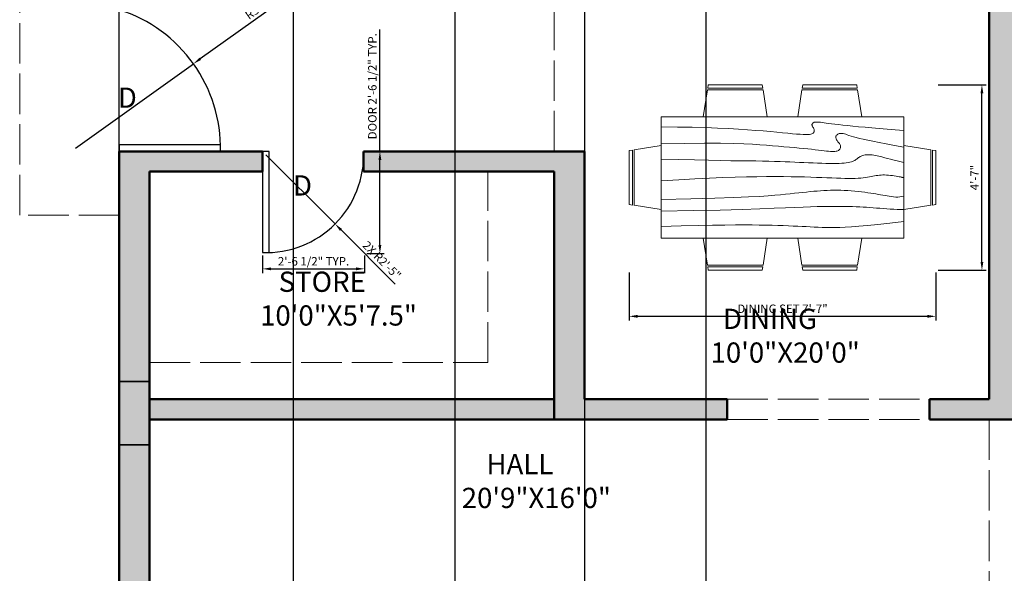
# Model space of a CAD drawing. Units: inches. Extents: x 5703 to 6226, y 10088 to 10813.
# Tile 3 of 5: x 5744 to 6036, y 10460 to 10624. Entities that reach past the tile are written whole.
import ezdxf

# ---------------------------------------------------------------- set-up
doc = ezdxf.new("R2010")
doc.units = ezdxf.units.IN
doc.linetypes.add('ACAD_ISO02W100', pattern=[15, 12, -3])
for name, color, linetype, lineweight in [('A-ANNO-DIMS', 2, 'Continuous', 18), ('A-ANNO-TEXT', 7, 'Continuous', 18), ('A-AREA-IDEN', 7, 'Continuous', 18), ('A-COLS', 7, 'Continuous', 35), ('A-COLS-PATT', 7, 'Continuous', 13), ('A-DOOR', 140, 'Continuous', 25), ('A-FURN', 8, 'Continuous', 18), ('A-WALL', 7, 'Continuous', 50), ('A-WALL-PATT', 9, 'Continuous', 13)]:
    doc.layers.add(name, color=color, linetype=linetype, lineweight=lineweight)
for name, color, linetype, lineweight, true_color in [('A-FLOR-CASE-OVHD', 30, 'ACAD_ISO02W100', 18, 0xf8991e), ('A-ROOF-OVHD', 30, 'ACAD_ISO02W100', 18, 0xf8991e), ('A-WALL-OVHD', 30, 'ACAD_ISO02W100', 18, 0xf8991e)]:
    doc.layers.add(name, color=color, linetype=linetype, lineweight=lineweight, true_color=true_color)
doc.styles.get("Standard").update_dxf_attribs({"font": 'arial.ttf'})
doc.dimstyles.new('ISO-25', dxfattribs={"dimtxt": 2.5, "dimasz": 2.5, "dimexe": 1.25, "dimexo": 0.625, "dimtad": 1, "dimlunit": 3, "dimtxsty": 'Standard', "dimcen": 2.5, "dimadec": 0, "dimazin": 0, "dimtfac": 1, "dimtmove": 0, "dimatfit": 3, "dimfxl": 1, "dimarcsym": 0})

# ---------------------------------------------------------------- blocks, each defined once
blk = doc.blocks.new('Dining Set - 36 x 72 in.')
for p, q in [((-22, 27.5), (-22.1562, 26.50042)), ((-5.8416, 26.5), (-22.1534, 26.5)), ((-22, 27.5), (-6, 27.5)), ((-5.8437, 26.49966), (-6, 27.5)), ((6, 27.5), (5.8438, 26.50042)), ((22.1584, 26.5), (5.8466, 26.5)), ((6, 27.5), (22, 27.5)), ((22.1563, 26.49966), (22, 27.5)), ((-22.2343, 26.00059), (-23.4847, 17.99762)), ((-22.2304, 26), (-5.7608, 26)), ((-4.5152, 17.99762), (-5.7655, 25.99926)), ((5.7657, 26.00059), (4.5153, 17.99762)), ((5.7696, 26), (22.2392, 26)), ((23.4848, 17.99762), (22.2345, 25.99926)), ((36, 18), (-36, 18)), ((-36, 18), (-36, -18)), ((36, -18), (36, 18)), ((-44.0006, 8.23428), (-35.9976, 9.48474)), ((44.0006, 8.23428), (35.9976, 9.48474)), ((-45.5, 8), (-44.5004, 8.15617)), ((-45.5, 8), (-45.5, -8)), ((-44.5, -8.15843), (-44.5, 8.15338)), ((-44, 8.23041), (-44, -8.23915)), ((44, 8.23041), (44, -8.23915)), ((44.5, -8.15843), (44.5, 8.15338)), ((45.5, 8), (44.5005, 8.15617)), ((45.5, 8), (45.5, -8)), ((-44.4997, -8.15631), (-45.5, -8)), ((-35.9976, -9.48476), (-43.9993, -8.2345)), ((35.9976, -9.48476), (43.9993, -8.2345)), ((44.4997, -8.15631), (45.5, -8)), ((-36, -18), (36, -18)), ((-22.2343, -26.0006), (-23.4847, -17.99762)), ((-4.5152, -17.99762), (-5.7655, -25.99928)), ((5.7657, -26.0006), (4.5153, -17.99762)), ((23.4848, -17.99762), (22.2345, -25.99928)), ((-22.2304, -26), (-5.7608, -26)), ((5.7696, -26), (22.2392, -26)), ((-22, -27.5), (-22.1562, -26.50044)), ((-5.8416, -26.5), (-22.1534, -26.5)), ((-22, -27.5), (-6, -27.5)), ((-5.8437, -26.49967), (-6, -27.5)), ((6, -27.5), (5.8438, -26.50044)), ((22.1584, -26.5), (5.8466, -26.5)), ((6, -27.5), (22, -27.5)), ((22.1563, -26.49967), (22, -27.5))]:
    blk.add_line(p, q)
for points in [[(-36, 15), (-31.1772, 14.97754), (-26.8079, 14.91406), (-22.8538, 14.81543), (-19.276, 14.6875), (-16.0362, 14.53613), (-13.0957, 14.36718), (-10.4159, 14.18652), (-7.9583, 14), (-5.6904, 13.81315), (-3.6035, 13.63021), (-1.6954, 13.45508), (0.0365, 13.29166), (1.5945, 13.14388), (2.9811, 13.01562), (4.1988, 12.9108), (5.25, 12.83333), (6.1393, 12.78613), (6.8802, 12.76823), (7.4883, 12.77767), (7.9792, 12.8125), (8.3685, 12.87077), (8.6719, 12.95052), (8.9049, 13.0498), (9.0833, 13.16666), (9.2205, 13.29899), (9.3216, 13.44401), (9.3895, 13.59879), (9.4271, 13.76041), (9.4373, 13.92594), (9.4232, 14.09245), (9.3875, 14.257), (9.3333, 14.41666), (9.2638, 14.56917), (9.1836, 14.71484), (9.0975, 14.85465), (9.0104, 14.98958), (8.9272, 15.1206), (8.8529, 15.2487), (8.7922, 15.37483), (8.75, 15.5), (8.7305, 15.62467), (8.7344, 15.74739), (8.7617, 15.86621), (8.8125, 15.97916), (8.8867, 16.08431), (8.9844, 16.17968), (9.1055, 16.26334), (9.25, 16.33333), (9.4189, 16.38802), (9.6172, 16.42708), (9.8506, 16.45052), (10.125, 16.45833), (10.4463, 16.45052), (10.8203, 16.42708), (11.2529, 16.38802), (11.75, 16.33333), (12.3184, 16.26318), (12.9694, 16.17838), (13.7151, 16.07991), (14.5677, 15.96875), (15.5395, 15.84586), (16.6426, 15.71224), (17.8893, 15.56884), (19.2917, 15.41666), (20.859, 15.25667), (22.5879, 15.08984), (24.4721, 14.91715), (26.5052, 14.73958), (28.6809, 14.5581), (30.9929, 14.3737), (33.4347, 14.18733), (36, 14)], [(-36, 10), (-28.9766, 10.14274), (-23.1725, 10.20442), (-18.4241, 10.19775), (-14.5677, 10.13541), (-11.4399, 10.03011), (-8.877, 9.89453), (-6.7154, 9.74137), (-4.7917, 9.58333), (-2.9698, 9.43082), (-1.2246, 9.28515), (0.4415, 9.14534), (2.026, 9.01041), (3.5266, 8.87939), (4.9408, 8.7513), (6.266, 8.62516), (7.5, 8.5), (8.6411, 8.37549), (9.6914, 8.2539), (10.6538, 8.13818), (11.5312, 8.03125), (12.3267, 7.93603), (13.043, 7.85547), (13.6831, 7.79248), (14.25, 7.75), (14.7471, 7.7303), (15.1797, 7.73307), (15.5537, 7.75732), (15.875, 7.80208), (16.1494, 7.86637), (16.3828, 7.94922), (16.5811, 8.04964), (16.75, 8.16666), (16.8944, 8.29915), (17.0143, 8.44531), (17.1089, 8.60319), (17.1771, 8.77083), (17.218, 8.94629), (17.2305, 9.1276), (17.2137, 9.31282), (17.1667, 9.5), (17.0895, 9.6875), (16.987, 9.875), (16.8649, 10.0625), (16.7292, 10.25), (16.5856, 10.4375), (16.4401, 10.625), (16.2985, 10.8125), (16.1667, 11), (16.05, 11.18733), (15.9518, 11.3737), (15.8752, 11.5581), (15.8229, 11.73958), (15.798, 11.91715), (15.8034, 12.08984), (15.842, 12.25667), (15.9167, 12.41666), (16.0295, 12.56836), (16.1784, 12.70833), (16.3605, 12.83268), (16.5729, 12.9375), (16.8127, 13.01888), (17.0768, 13.07291), (17.3625, 13.0957), (17.6667, 13.08333), (17.9894, 13.03312), (18.3418, 12.94726), (18.7382, 12.82918), (19.1927, 12.68229), (19.7195, 12.51001), (20.3327, 12.31575), (21.0465, 12.10294), (21.875, 11.875), (22.8357, 11.63354), (23.959, 11.37304), (25.2786, 11.08618), (26.8282, 10.76562), (28.6414, 10.40405), (30.752, 9.99414), (33.1936, 9.52856), (36, 9)], [(-36, 5.5), (-30.7157, 5.3348), (-26.069, 5.20963), (-21.9946, 5.11767), (-18.4271, 5.05208), (-15.3009, 5.00602), (-12.5508, 4.97265), (-10.1112, 4.94515), (-7.9167, 4.91666), (-5.909, 4.88167), (-4.0586, 4.83984), (-2.3429, 4.79215), (-0.7396, 4.73958), (0.7739, 4.6831), (2.22, 4.6237), (3.6213, 4.56233), (5, 4.5), (6.373, 4.43782), (7.7344, 4.3776), (9.0723, 4.32129), (10.375, 4.27083), (11.6309, 4.22819), (12.8281, 4.19531), (13.9551, 4.17415), (15, 4.16666), (15.954, 4.17448), (16.819, 4.19791), (17.6001, 4.23698), (18.3021, 4.29166), (18.9299, 4.36198), (19.4883, 4.44791), (19.9823, 4.54948), (20.4167, 4.66666), (20.7969, 4.79899), (21.1302, 4.94401), (21.4245, 5.09879), (21.6875, 5.26041), (21.9271, 5.42594), (22.1511, 5.59245), (22.3672, 5.757), (22.5834, 5.91666), (22.8065, 6.06868), (23.0404, 6.21093), (23.2879, 6.34147), (23.5521, 6.45833), (23.8358, 6.55957), (24.142, 6.64323), (24.4735, 6.70735), (24.8334, 6.75), (25.2235, 6.76969), (25.642, 6.76692), (26.0858, 6.74267), (26.5521, 6.69791), (27.0379, 6.63362), (27.5404, 6.55078), (28.0565, 6.45036), (28.5834, 6.33333), (29.1242, 6.19987), (29.7071, 6.04687), (30.3661, 5.87044), (31.1354, 5.66666), (32.0493, 5.43164), (33.142, 5.16146), (34.4475, 4.85221), (36, 4.5)], [(-36, -1), (-30.7915, -0.6591), (-26.0195, -0.38216), (-21.6519, -0.16284), (-17.6563, 0.00521), (-14.0005, 0.12833), (-10.6523, 0.21289), (-7.5796, 0.26522), (-4.75, 0.29166), (-2.134, 0.29793), (0.2878, 0.28711), (2.5317, 0.26163), (4.6146, 0.22396), (6.5529, 0.17651), (8.3633, 0.12174), (10.0623, 0.06209), (11.6667, 0), (13.1899, -0.06201), (14.6341, -0.1211), (15.9982, -0.17432), (17.2813, -0.21875), (18.4823, -0.25147), (19.6003, -0.26953), (20.6343, -0.27002), (21.5834, -0.25), (22.4481, -0.20768), (23.2357, -0.14584), (23.9549, -0.06836), (24.6146, 0.02083), (25.2235, 0.11784), (25.7904, 0.21875), (26.3241, 0.31966), (26.8334, 0.41666), (27.3265, 0.50618), (27.8099, 0.58593), (28.2894, 0.65397), (28.7709, 0.70833), (29.2601, 0.74707), (29.763, 0.76823), (30.2855, 0.76985), (30.8334, 0.75), (31.4088, 0.70784), (31.9994, 0.64713), (32.589, 0.57275), (33.1615, 0.48958), (33.7008, 0.4025), (34.1908, 0.3164), (34.6153, 0.23616), (34.9584, 0.16666), (35.2099, 0.11165), (35.3848, 0.07031), (35.504, 0.04069), (35.5886, 0.02083), (35.6594, 0.00879), (35.7377, 0.0026), (35.8442, 0.00032), (36, 0)], [(-36, -6.5), (-27.1843, -6.31267), (-20.084, -6.1263), (-14.469, -5.9419), (-10.1094, -5.76042), (-6.7752, -5.58285), (-4.2363, -5.41016), (-2.2629, -5.24333), (-0.625, -5.08334), (0.8708, -4.93099), (2.2715, -4.78646), (3.5872, -4.64974), (4.8281, -4.52084), (6.0046, -4.39974), (7.127, -4.28646), (8.2053, -4.18099), (9.25, -4.08334), (10.2705, -3.99382), (11.2734, -3.91407), (12.2647, -3.84603), (13.25, -3.79167), (14.2354, -3.75293), (15.2266, -3.73177), (16.2295, -3.73015), (17.25, -3.75), (18.2912, -3.79248), (19.3451, -3.85547), (20.4009, -3.93604), (21.4479, -4.03125), (22.4754, -4.13819), (23.4727, -4.25391), (24.4289, -4.37549), (25.3334, -4.5), (26.1785, -4.62492), (26.9694, -4.74935), (27.7145, -4.87281), (28.4219, -4.99479), (29.1, -5.11483), (29.7572, -5.23242), (30.4016, -5.34709), (31.0417, -5.45834), (31.6837, -5.56437), (32.3262, -5.65821), (32.9658, -5.73153), (33.599, -5.77604), (34.2224, -5.78345), (34.8327, -5.74545), (35.4264, -5.65373), (36, -5.5)], [(-36, -10), (-26.4022, -9.81299), (-18.4675, -9.62891), (-11.9839, -9.45069), (-6.7396, -9.28125), (-2.5226, -9.12354), (0.8789, -8.98047), (3.6769, -8.85498), (6.0833, -8.75), (8.2767, -8.66765), (10.3021, -8.60677), (12.1712, -8.56543), (13.8958, -8.54167), (15.4876, -8.53353), (16.9583, -8.53907), (18.3197, -8.55632), (19.5834, -8.58334), (20.7616, -8.61841), (21.8685, -8.66081), (22.9188, -8.71004), (23.9271, -8.76563), (24.9081, -8.82707), (25.8763, -8.89388), (26.8465, -8.96558), (27.8334, -9.04167), (28.8474, -9.12118), (29.8828, -9.20117), (30.93, -9.27824), (31.9792, -9.34896), (33.0205, -9.40991), (34.0443, -9.45768), (35.0407, -9.48885), (36, -9.5)], [(-36, -14.5), (-30.0881, -14.33513), (-25.0332, -14.21224), (-20.7312, -14.12647), (-17.0781, -14.07292), (-13.97, -14.04671), (-11.3027, -14.04297), (-8.9724, -14.05681), (-6.875, -14.08334), (-4.9224, -14.11833), (-3.0905, -14.16016), (-1.3709, -14.20785), (0.2448, -14.26042), (1.7647, -14.3169), (3.1973, -14.3763), (4.5507, -14.43767), (5.8333, -14.5), (7.0554, -14.5621), (8.235, -14.62175), (9.3922, -14.67652), (10.5469, -14.72396), (11.7192, -14.76164), (12.929, -14.78711), (14.1965, -14.79794), (15.5417, -14.79167), (16.9933, -14.76424), (18.6152, -14.70508), (20.4804, -14.60197), (22.6615, -14.44271), (25.2312, -14.21509), (28.2624, -13.9069), (31.8277, -13.50594), (36, -13)]]:
    blk.add_lwpolyline(points)
blk = doc.blocks.new('DOOR-SWING-30')
for p, q in [((0, 30.02), (0, 0.02)), ((2, 30.02), (0, 30.02)), ((2, 0.02), (2, 30.02)), ((0, 0.02), (2, 0.02))]:
    blk.add_line(p, q)
blk.add_arc((1, 29.02), 29.02, 268.0251, 1.9749)
blk = doc.blocks.new('*D26')
at = {"layer": 'A-ANNO-DIMS', "color": 0, "lineweight": -2, "transparency": 16777216}
for p, q in [((5850.48, 10584.87), (5850.48, 10621.01)), ((5846.57, 10584.87), (5851.73, 10584.87)), ((5850.48, 10557.09), (5850.48, 10582.37)), ((5846.57, 10554.59), (5851.73, 10554.59))]:
    blk.add_line(p, q, dxfattribs=at)
at = {"layer": 'A-ANNO-DIMS', "color": 0, "transparency": 16777216}
for points in [[(5850.07, 10582.37), (5850.9, 10582.37), (5850.48, 10584.87)], [(5850.07, 10557.09), (5850.9, 10557.09), (5850.48, 10554.59)]]:
    blk.add_solid(points, dxfattribs=at)
at = {"layer": 'Defpoints', "color": 0, "transparency": 16777216}
for p in [(5845.94, 10584.87), (5850.48, 10584.87), (5845.94, 10554.59)]:
    blk.add_point(p, dxfattribs=at)
at = {"layer": 'A-ANNO-DIMS', "color": 0, "transparency": 16777216, "insert": (5848.57, 10604.19), "char_height": 2.5, "attachment_point": 5, "rotation": 90}
blk.add_mtext('DOOR 2\'-6 1/2" TYP.', dxfattribs=at)
blk = doc.blocks.new('*D27')
at = {"layer": 'A-ANNO-DIMS', "color": 0, "lineweight": -2, "transparency": 16777216}
for p, q in [((5815.67, 10553.97), (5815.67, 10548.8)), ((5845.94, 10553.97), (5845.94, 10548.8)), ((5818.17, 10550.05), (5843.44, 10550.05))]:
    blk.add_line(p, q, dxfattribs=at)
at = {"layer": 'A-ANNO-DIMS', "color": 0, "transparency": 16777216}
for points in [[(5818.17, 10550.47), (5818.17, 10549.63), (5815.67, 10550.05)], [(5843.44, 10550.47), (5843.44, 10549.63), (5845.94, 10550.05)]]:
    blk.add_solid(points, dxfattribs=at)
at = {"layer": 'Defpoints', "color": 0, "transparency": 16777216}
for p in [(5815.67, 10554.59), (5845.94, 10554.59), (5845.94, 10550.05)]:
    blk.add_point(p, dxfattribs=at)
at = {"layer": 'A-ANNO-DIMS', "color": 0, "transparency": 16777216, "insert": (5830.8, 10551.97), "char_height": 2.5, "attachment_point": 5}
blk.add_mtext('2\'-6 1/2" TYP.', dxfattribs=at)
blk = doc.blocks.new('*D32')
at = {"layer": 'A-ANNO-DIMS', "color": 0, "lineweight": -2, "transparency": 16777216}
for p, q in [((5924.39, 10549), (5924.39, 10534.72)), ((6015.39, 10549), (6015.39, 10534.72)), ((5926.89, 10535.97), (6012.89, 10535.97))]:
    blk.add_line(p, q, dxfattribs=at)
at = {"layer": 'A-ANNO-DIMS', "color": 0, "transparency": 16777216}
for points in [[(5926.89, 10536.39), (5926.89, 10535.55), (5924.39, 10535.97)], [(6012.89, 10536.39), (6012.89, 10535.55), (6015.39, 10535.97)]]:
    blk.add_solid(points, dxfattribs=at)
at = {"layer": 'Defpoints', "color": 0, "transparency": 16777216}
for p in [(5924.39, 10549.62), (6015.39, 10549.62), (6015.39, 10535.97)]:
    blk.add_point(p, dxfattribs=at)
at = {"layer": 'A-ANNO-DIMS', "color": 0, "transparency": 16777216, "insert": (5969.89, 10537.89), "char_height": 2.5, "attachment_point": 5}
blk.add_mtext('DINING SET 7\'-7"', dxfattribs=at)
blk = doc.blocks.new('*D33')
at = {"layer": 'A-ANNO-DIMS', "color": 0, "lineweight": -2, "transparency": 16777216}
for p, q in [((6016.02, 10604.62), (6030.29, 10604.62)), ((6029.04, 10552.12), (6029.04, 10602.12)), ((6016.02, 10549.62), (6030.29, 10549.62))]:
    blk.add_line(p, q, dxfattribs=at)
at = {"layer": 'A-ANNO-DIMS', "color": 0, "transparency": 16777216}
for points in [[(6028.62, 10602.12), (6029.46, 10602.12), (6029.04, 10604.62)], [(6028.62, 10552.12), (6029.46, 10552.12), (6029.04, 10549.62)]]:
    blk.add_solid(points, dxfattribs=at)
at = {"layer": 'Defpoints', "color": 0, "transparency": 16777216}
for p in [(6015.39, 10604.62), (6029.04, 10604.62), (6015.39, 10549.62)]:
    blk.add_point(p, dxfattribs=at)
at = {"layer": 'A-ANNO-DIMS', "color": 0, "transparency": 16777216, "insert": (6027.17, 10577.12), "char_height": 2.5, "attachment_point": 5, "rotation": 90}
blk.add_mtext('4\'-7"', dxfattribs=at)
blk = doc.blocks.new('*D40')
at = {"layer": 'A-ANNO-DIMS', "color": 0, "lineweight": -2, "transparency": 16777216}
for p, q in [((5911.18, 10644.24), (5911.18, 10088.29)), ((5947.18, 10644.24), (5947.18, 10088.29)), ((5913.68, 10089.54), (5944.68, 10089.54))]:
    blk.add_line(p, q, dxfattribs=at)
at = {"layer": 'A-ANNO-DIMS', "color": 0, "transparency": 16777216}
for points in [[(5913.68, 10089.96), (5913.68, 10089.12), (5911.18, 10089.54)], [(5944.68, 10089.96), (5944.68, 10089.12), (5947.18, 10089.54)]]:
    blk.add_solid(points, dxfattribs=at)
at = {"layer": 'Defpoints', "color": 0, "transparency": 16777216}
for p in [(5911.18, 10644.87), (5947.18, 10644.87), (5947.18, 10089.54)]:
    blk.add_point(p, dxfattribs=at)
at = {"layer": 'A-ANNO-DIMS', "color": 0, "transparency": 16777216, "insert": (5929.18, 10091.44), "char_height": 2.5, "attachment_point": 5}
blk.add_mtext('3\'-0"', dxfattribs=at)
blk = doc.blocks.new('*D47')
at = {"layer": 'A-ANNO-DIMS', "color": 0, "lineweight": -2, "transparency": 16777216}
for p, q in [((5824.85, 10313.99), (5824.85, 10785.97)), ((5827.35, 10784.72), (5870.35, 10784.72)), ((5872.85, 10313.99), (5872.85, 10785.97))]:
    blk.add_line(p, q, dxfattribs=at)
at = {"layer": 'A-ANNO-DIMS', "color": 0, "transparency": 16777216}
for points in [[(5827.35, 10785.14), (5827.35, 10784.3), (5824.85, 10784.72)], [(5870.35, 10785.14), (5870.35, 10784.3), (5872.85, 10784.72)]]:
    blk.add_solid(points, dxfattribs=at)
at = {"layer": 'Defpoints', "color": 0, "transparency": 16777216}
for p in [(5872.85, 10784.72), (5824.85, 10313.37), (5872.85, 10313.37)]:
    blk.add_point(p, dxfattribs=at)
at = {"layer": 'A-ANNO-DIMS', "color": 0, "transparency": 16777216, "insert": (5848.85, 10786.62), "char_height": 2.5, "attachment_point": 5}
blk.add_mtext('4\'-0"', dxfattribs=at)
blk = doc.blocks.new('*D48')
at = {"layer": 'A-ANNO-DIMS', "color": 0, "lineweight": -2, "transparency": 16777216}
for p, q in [((5773.18, 10304.99), (5773.18, 10785.97)), ((5775.68, 10784.72), (5822.35, 10784.72)), ((5824.85, 10304.99), (5824.85, 10785.97))]:
    blk.add_line(p, q, dxfattribs=at)
at = {"layer": 'A-ANNO-DIMS', "color": 0, "transparency": 16777216}
for points in [[(5775.68, 10785.14), (5775.68, 10784.3), (5773.18, 10784.72)], [(5822.35, 10785.14), (5822.35, 10784.3), (5824.85, 10784.72)]]:
    blk.add_solid(points, dxfattribs=at)
at = {"layer": 'Defpoints', "color": 0, "transparency": 16777216}
for p in [(5824.85, 10784.72), (5773.18, 10304.37), (5824.85, 10304.37)]:
    blk.add_point(p, dxfattribs=at)
at = {"layer": 'A-ANNO-DIMS', "color": 0, "transparency": 16777216, "insert": (5799.01, 10786.64), "char_height": 2.5, "attachment_point": 5}
blk.add_mtext('4\'-3 1/2"', dxfattribs=at)
blk = doc.blocks.new('*D58')
at = {"layer": 'A-ANNO-DIMS', "color": 0, "lineweight": -2, "transparency": 16777216}
for p, q in [((5820.36, 10628.86), (5797.21, 10612.32)), ((5760.18, 10585.87), (5795.18, 10610.87))]:
    blk.add_line(p, q, dxfattribs=at)
at = {"layer": 'A-ANNO-DIMS', "color": 0, "transparency": 16777216}
blk.add_solid([(5796.97, 10612.66), (5797.45, 10611.98), (5795.18, 10610.87)], dxfattribs=at)
at = {"layer": 'Defpoints', "color": 0, "transparency": 16777216}
for p in [(5795.18, 10610.87), (5760.18, 10585.87)]:
    blk.add_point(p, dxfattribs=at)
at = {"layer": 'A-ANNO-DIMS', "color": 0, "transparency": 16777216, "insert": (5815.07, 10627.42), "char_height": 2.5, "attachment_point": 5, "rotation": 35.5383}
blk.add_mtext('R3\'-7"', dxfattribs=at)
blk = doc.blocks.new('*D63')
at = {"layer": 'A-ANNO-DIMS', "color": 0, "lineweight": -2, "transparency": 16777216}
for p, q in [((5816.67, 10583.87), (5837.18, 10563.35)), ((5855.05, 10545.49), (5838.95, 10561.58))]:
    blk.add_line(p, q, dxfattribs=at)
at = {"layer": 'A-ANNO-DIMS', "color": 0, "transparency": 16777216}
blk.add_solid([(5839.25, 10561.88), (5838.66, 10561.29), (5837.18, 10563.35)], dxfattribs=at)
at = {"layer": 'Defpoints', "color": 0, "transparency": 16777216}
for p in [(5816.67, 10583.87), (5837.18, 10563.35)]:
    blk.add_point(p, dxfattribs=at)
at = {"layer": 'A-ANNO-DIMS', "color": 0, "transparency": 16777216, "insert": (5850.84, 10552.38), "char_height": 2.5, "attachment_point": 5, "rotation": 314.9996}
blk.add_mtext('2X R2\'-5"', dxfattribs=at)

msp = doc.modelspace()

# ---------------------------------------------------------------- hatches: boundary and pattern name
at = {"layer": 'A-COLS-PATT'}
h = msp.add_hatch(color=256, dxfattribs=at)
h.dxf.hatch_style = 1
h.paths.add_polyline_path([(5788.176, 10725.869), (5773.176, 10725.869), (5773.176, 10716.869), (5788.176, 10716.869)])
h.paths.add_polyline_path([(5782.176, 10516.684), (5773.176, 10516.684), (5773.176, 10497.849), (5782.176, 10497.849)])
h.paths.add_polyline_path([(5782.176, 10319.369), (5773.176, 10319.369), (5773.176, 10304.369), (5782.176, 10304.369)])
h.paths.add_polyline_path([(5960.955, 10313.369), (5953.525, 10313.369), (5953.525, 10304.369), (5960.955, 10304.369)])
h.paths.add_polyline_path([(6040.176, 10314.869), (6031.176, 10314.869), (6031.176, 10304.369), (6040.176, 10304.369)])
h.paths.add_polyline_path([(6181.176, 10198.545), (6172.176, 10198.545), (6172.176, 10178.369), (6181.176, 10178.369)])
h.paths.add_polyline_path([(6181.176, 10505.369), (6172.176, 10505.369), (6172.176, 10492.633), (6181.176, 10492.633)])
h.paths.add_polyline_path([(6181.176, 10725.869), (6166.176, 10725.869), (6166.176, 10716.869), (6181.176, 10716.869)])
at = {"layer": 'A-WALL-PATT'}
h = msp.add_hatch(color=256, dxfattribs=at)
h.dxf.hatch_style = 1
h.paths.add_polyline_path([(6057.982, 10725.869), (6040.176, 10725.869), (6040.176, 10749.869), (5999.271, 10749.869), (5999.271, 10740.869), (6031.176, 10740.869), (6031.176, 10716.869), (6031.176, 10511.369), (6013.525, 10511.369), (6013.525, 10505.369), (6048.161, 10505.369), (6048.161, 10511.369), (6040.176, 10511.369), (6040.176, 10716.869), (6057.982, 10716.869)])
h.paths.add_polyline_path([(6166.176, 10725.869), (6093.982, 10725.869), (6093.982, 10716.869), (6166.176, 10716.869)])
h.paths.add_polyline_path([(6181.176, 10716.869), (6172.176, 10716.869), (6172.176, 10511.369), (6132.161, 10511.369, -0.0172363), (6132.161, 10509.369), (6132.161, 10505.369), (6181.176, 10505.369)])
h.paths.add_polyline_path([(6181.176, 10468.633), (6172.176, 10468.633), (6172.176, 10451.369), (6098.676, 10451.369), (6098.676, 10505.369), (6102.161, 10505.369), (6102.161, 10511.369), (6090.161, 10511.369), (6090.161, 10507.369, -0.0121933), (6090.161, 10505.369), (6092.676, 10505.369), (6092.676, 10451.369), (6085.668, 10451.369), (6085.668, 10445.369), (6092.676, 10445.369), (6172.176, 10445.369), (6172.176, 10342.529), (6181.176, 10342.529)])
h.paths.add_polyline_path([(6181.176, 10282.529), (6172.176, 10282.529), (6172.176, 10253.369), (6092.676, 10253.369), (6092.676, 10247.369), (6094.176, 10247.369), (6094.176, 10238.954), (6100.176, 10238.954), (6100.176, 10247.369), (6172.176, 10247.369), (6172.176, 10234.545), (6181.176, 10234.545)])
h.paths.add_polyline_path([(6172.176, 10187.369), (6100.176, 10187.369), (6100.176, 10220.954), (6096.176, 10220.954, -0.0293864), (6094.176, 10220.954), (6094.176, 10178.369), (6172.176, 10178.369)])
h.paths.add_polyline_path([(6050.745, 10187.369), (6040.176, 10187.369), (6040.176, 10178.369), (6050.745, 10178.369)])
h.paths.add_polyline_path([(6040.176, 10187.369), (6031.176, 10187.369), (6031.176, 10178.369), (6040.176, 10178.369)])
h.paths.add_polyline_path([(6040.176, 10304.369), (6031.176, 10304.369), (6031.176, 10187.369), (6040.176, 10187.369)])
h.paths.add_polyline_path([(6040.176, 10393.328), (6031.176, 10393.328), (6031.176, 10314.869), (6040.176, 10314.869)])
h.paths.add_polyline_path([(6040.176, 10445.369), (6046.458, 10445.369), (6046.458, 10451.369), (6031.176, 10451.369), (6031.176, 10408.328), (6040.176, 10408.328)])
h.paths.add_polyline_path([(5911.176, 10584.869), (5845.666, 10584.869, -0.0172363), (5845.666, 10582.869), (5845.666, 10578.869), (5902.176, 10578.869), (5902.176, 10505.369), (5953.525, 10505.369), (5953.525, 10511.369), (5911.176, 10511.369)])
h.paths.add_polyline_path([(5902.176, 10511.369), (5782.176, 10511.369), (5782.176, 10505.369), (5902.176, 10505.369)])
h.paths.add_polyline_path([(5782.176, 10578.869), (5815.666, 10578.869), (5815.666, 10584.869), (5773.176, 10584.869), (5773.176, 10516.684), (5782.176, 10516.684)])
h.paths.add_polyline_path([(5782.176, 10497.849), (5773.176, 10497.849), (5773.176, 10438.429), (5782.176, 10438.429)])
h.paths.add_polyline_path([(5782.176, 10378.429), (5773.176, 10378.429), (5773.176, 10319.369), (5782.176, 10319.369)])
h.paths.add_polyline_path([(5824.846, 10313.369), (5782.176, 10313.369), (5782.176, 10304.369), (5824.846, 10304.369)])
h.paths.add_polyline_path([(5953.525, 10313.369), (5872.846, 10313.369), (5872.846, 10304.369), (5953.525, 10304.369)])

# ---------------------------------------------------------------- linework, layer by layer
at = {"layer": 'A-COLS'}
for p, q in [((5782.176, 10516.684), (5773.176, 10516.684)), ((5782.176, 10497.849), (5773.176, 10497.849))]:
    msp.add_line(p, q, dxfattribs=at)
at = {"layer": 'A-DOOR'}
for p, q in [((5803.176, 10586.869), (5773.176, 10586.869)), ((5773.176, 10586.869), (5773.176, 10584.869)), ((5803.176, 10584.869), (5803.176, 10586.869)), ((5773.176, 10584.869), (5803.176, 10584.869))]:
    msp.add_line(p, q, dxfattribs=at)
msp.add_arc((5760.176, 10585.869), 43.012, 358.66778, 72.40758, dxfattribs=at)
at = {"layer": 'A-FLOR-CASE-OVHD'}
for p, q in [((5882.481, 10522.278), (5882.481, 10578.869)), ((5782.176, 10522.278), (5882.481, 10522.278))]:
    msp.add_line(p, q, dxfattribs=at)
at = {"layer": 'A-ROOF-OVHD'}
for p, q in [((5743.649, 10565.956), (5743.649, 10711.167)), ((5773.176, 10565.956), (5743.649, 10565.956))]:
    msp.add_line(p, q, dxfattribs=at)
at = {"layer": 'A-WALL'}
for p, q in [((6031.176, 10511.369), (6031.176, 10716.869)), ((5773.176, 10584.869), (5815.666, 10584.869)), ((5773.176, 10438.429), (5773.176, 10584.869)), ((5815.666, 10584.869), (5815.666, 10578.869)), ((5845.666, 10584.869), (5845.666, 10578.869)), ((5845.666, 10584.869), (5911.176, 10584.869)), ((5911.176, 10511.369), (5911.176, 10584.869)), ((5782.176, 10578.869), (5815.666, 10578.869)), ((5782.176, 10438.429), (5782.176, 10578.869)), ((5845.666, 10578.869), (5902.176, 10578.869)), ((5902.176, 10505.369), (5902.176, 10578.869)), ((5782.176, 10511.369), (5902.176, 10511.369)), ((5911.176, 10511.369), (5953.525, 10511.369)), ((5953.525, 10511.369), (5953.525, 10505.369)), ((6013.525, 10511.369), (6013.525, 10505.369)), ((6013.525, 10511.369), (6031.176, 10511.369)), ((5782.176, 10505.369), (5953.525, 10505.369)), ((6013.525, 10505.369), (6048.161, 10505.369))]:
    msp.add_line(p, q, dxfattribs=at)
at = {"layer": 'A-WALL-OVHD'}
for p, q in [((5902.176, 10584.869), (5902.176, 10626.869)), ((5911.176, 10584.869), (5911.176, 10626.869)), ((5953.525, 10511.369), (6013.525, 10511.369)), ((5953.525, 10505.369), (6013.525, 10505.369)), ((6031.176, 10505.369), (6031.176, 10451.369))]:
    msp.add_line(p, q, dxfattribs=at)

# ---------------------------------------------------------------- block references
at = {"layer": 'A-DOOR'}
msp.add_blockref('DOOR-SWING-30', (5815.666, 10554.852), dxfattribs=at)
at = {"layer": 'A-FURN'}
msp.add_blockref('Dining Set - 36 x 72 in.', (5969.892, 10577.12), dxfattribs=at)

# ---------------------------------------------------------------- texts
at = {"layer": 'A-ANNO-TEXT', "char_height": 6, "attachment_point": 1}
for insert in [(5770.925, 10603.817), (5822.869, 10577.781)]:
    msp.add_mtext_dynamic_manual_height_columns(' D', width=71.13425, gutter_width=12.5, heights=[0], dxfattribs=dict(at, insert=insert))
at = {"layer": 'A-AREA-IDEN', "char_height": 6, "attachment_point": 1}
for s, heights, insert in [('   STORE\\P10\'0"X5\'7.5"', [0], (5814.946, 10549.224)), ('  DINING\\P10\'0"X20\'0"', [0], (5948.556, 10538.216)), ('     HALL\\P 20\'9"X16\'0"', [16.229], (5872.923, 10495.117))]:
    msp.add_mtext_dynamic_manual_height_columns(s, width=71.13425, gutter_width=12.5, heights=heights, dxfattribs=dict(at, insert=insert))

# ---------------------------------------------------------------- dimensions: what is measured, and where the dimension line sits
at = {"layer": 'A-ANNO-DIMS'}
for base, p1, p2, picture, middle in [((5824.846, 10784.719), (5773.176, 10304.369), (5824.846, 10304.369), '*D48', (5799.011, 10786.637)), ((5872.846, 10784.719), (5824.846, 10313.369), (5872.846, 10313.369), '*D47', (5848.846, 10786.62)), ((5947.176, 10089.539), (5911.176, 10644.869), (5947.176, 10644.869), '*D40', (5929.176, 10091.442))]:
    dim = msp.add_linear_dim(base=base, p1=p1, p2=p2, dimstyle='ISO-25', override={"dimdec": 1, "dimlfac": 1, "dimrnd": 0, "dimzin": 1, "dimdsep": 46, "dimlunit": 4, "dimfrac": 2}, dxfattribs=at)
    dim.commit()
    dim.dimension.update_dxf_attribs({"geometry": picture, "text_midpoint": middle})
dim = msp.add_radius_dim(center=(5760.176, 10585.869), mpoint=(5795.176, 10610.869), dimstyle='ISO-25', override={"dimdec": 1, "dimlfac": 1, "dimrnd": 0, "dimzin": 1, "dimdsep": 46, "dimlunit": 4, "dimfrac": 2}, dxfattribs=at)
dim.commit()
dim.dimension.update_dxf_attribs({"geometry": '*D58', "text_midpoint": (5816.176, 10625.869), "dimtype": 164})
dim = msp.add_linear_dim(base=(5850.484, 10584.869), p1=(5845.943, 10554.591), p2=(5845.943, 10584.869), angle=90, text='DOOR <> TYP.', dimstyle='ISO-25', override={"dimdec": 1, "dimlfac": 1, "dimrnd": 0, "dimzin": 1, "dimdsep": 46, "dimlunit": 4, "dimfrac": 2}, dxfattribs=at)
dim.commit()
dim.dimension.update_dxf_attribs({"geometry": '*D26', "text_midpoint": (5848.566, 10604.187)})
dim = msp.add_linear_dim(base=(6029.042, 10604.62), p1=(6015.392, 10549.62), p2=(6015.392, 10604.62), angle=90, dimstyle='ISO-25', override={"dimdec": 1, "dimlfac": 1, "dimrnd": 0, "dimzin": 1, "dimdsep": 46, "dimlunit": 4, "dimfrac": 2}, dxfattribs=at)
dim.commit()
dim.dimension.update_dxf_attribs({"geometry": '*D33', "text_midpoint": (6027.167, 10577.12)})
dim = msp.add_radius_dim(center=(5816.666, 10583.869), mpoint=(5837.184, 10563.35), text='2X <>', dimstyle='ISO-25', override={"dimdec": 1, "dimlfac": 1, "dimrnd": 0, "dimzin": 1, "dimdsep": 46, "dimlunit": 4, "dimfrac": 2}, dxfattribs=at)
dim.commit()
dim.dimension.update_dxf_attribs({"geometry": '*D63', "text_midpoint": (5849.495, 10551.039), "dimtype": 164})
for base, p1, p2, text, picture, middle in [((5845.943, 10550.05), (5815.666, 10554.591), (5845.943, 10554.591), '<> TYP.', '*D27', (5830.804, 10551.968)), ((6015.392, 10535.97), (5924.392, 10549.62), (6015.392, 10549.62), 'DINING SET <>', '*D32', (5969.892, 10537.888))]:
    dim = msp.add_linear_dim(base=base, p1=p1, p2=p2, text=text, dimstyle='ISO-25', override={"dimdec": 1, "dimlfac": 1, "dimrnd": 0, "dimzin": 1, "dimdsep": 46, "dimlunit": 4, "dimfrac": 2}, dxfattribs=at)
    dim.commit()
    dim.dimension.update_dxf_attribs({"geometry": picture, "text_midpoint": middle})

doc.saveas('drawing.dxf')
